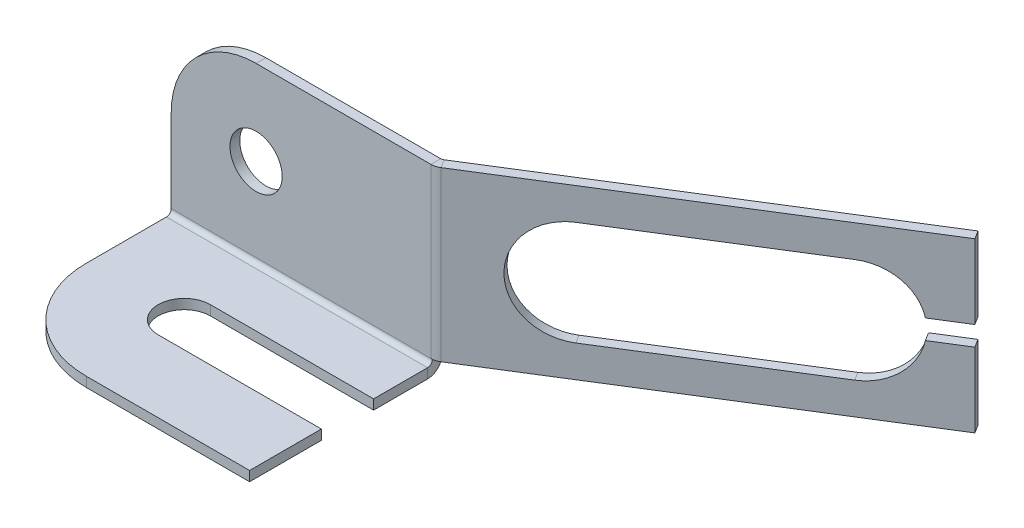
ISO-10303-21;
HEADER;
FILE_DESCRIPTION(('STEP AP214'),'2;1');
FILE_NAME('part.step','',(''),(''),'','','');
FILE_SCHEMA(('AUTOMOTIVE_DESIGN { 1 0 10303 214 1 1 1 1 }'));
ENDSEC;
DATA;
#1=APPLICATION_CONTEXT('core data for automotive mechanical design processes');
#2=APPLICATION_PROTOCOL_DEFINITION('international standard','automotive_design',2000,#1);
#3=PRODUCT_CONTEXT('',#1,'mechanical');
#4=PRODUCT('Part','Part','',(#3));
#5=PRODUCT_RELATED_PRODUCT_CATEGORY('part','',(#4));
#6=PRODUCT_DEFINITION_FORMATION('','',#4);
#7=PRODUCT_DEFINITION_CONTEXT('part definition',#1,'design');
#8=PRODUCT_DEFINITION('design','',#6,#7);
#9=PRODUCT_DEFINITION_SHAPE('','',#8);
#10=(LENGTH_UNIT() NAMED_UNIT(*) SI_UNIT(.MILLI.,.METRE.));
#11=(NAMED_UNIT(*) PLANE_ANGLE_UNIT() SI_UNIT($,.RADIAN.));
#12=(NAMED_UNIT(*) SI_UNIT($,.STERADIAN.) SOLID_ANGLE_UNIT());
#13=UNCERTAINTY_MEASURE_WITH_UNIT(LENGTH_MEASURE(1.E-05),#10,'distance_accuracy_value','');
#14=(GEOMETRIC_REPRESENTATION_CONTEXT(3) GLOBAL_UNCERTAINTY_ASSIGNED_CONTEXT((#13)) GLOBAL_UNIT_ASSIGNED_CONTEXT((#10,
#11,#12)) REPRESENTATION_CONTEXT('',''));
#15=CARTESIAN_POINT('',(0.,0.,0.));
#16=DIRECTION('',(0.,0.,1.));
#17=DIRECTION('',(1.,0.,0.));
#18=AXIS2_PLACEMENT_3D('',#15,#16,#17);
#19=CARTESIAN_POINT('',(91.3130038480239,0.736599999999992,-31.795155853992));
#20=DIRECTION('',(0.848048096156429,0.,-0.5299192642332));
#21=DIRECTION('',(-0.5299192642332,0.,-0.848048096156429));
#22=AXIS2_PLACEMENT_3D('',#19,#20,#21);
#23=PLANE('',#22);
#24=DIRECTION('',(0.5299192642332,0.,0.848048096156429));
#25=VECTOR('',#24,1.);
#26=CARTESIAN_POINT('',(91.3130038480239,15.1183,-31.795155853992));
#27=LINE('',#26,#25);
#28=CARTESIAN_POINT('',(90.5181249516741,15.1183,-33.0672279982266));
#29=VERTEX_POINT('',#28);
#30=CARTESIAN_POINT('',(91.3130038480239,15.1183,-31.795155853992));
#31=VERTEX_POINT('',#30);
#32=EDGE_CURVE('E463',#29,#31,#27,.T.);
#33=ORIENTED_EDGE('',*,*,#32,.F.);
#34=DIRECTION('',(0.,-1.,0.));
#35=VECTOR('',#34,1.);
#36=CARTESIAN_POINT('',(90.5181249516741,0.736599999999992,-33.0672279982266));
#37=LINE('',#36,#35);
#38=CARTESIAN_POINT('',(90.5181249516741,26.5,-33.0672279982266));
#39=VERTEX_POINT('',#38);
#40=EDGE_CURVE('E284',#39,#29,#37,.T.);
#41=ORIENTED_EDGE('',*,*,#40,.F.);
#42=DIRECTION('',(-0.5299192642332,0.,-0.848048096156429));
#43=VECTOR('',#42,1.);
#44=CARTESIAN_POINT('',(91.3130038480239,26.5,-31.795155853992));
#45=LINE('',#44,#43);
#46=CARTESIAN_POINT('',(91.3130038480239,26.5,-31.795155853992));
#47=VERTEX_POINT('',#46);
#48=EDGE_CURVE('E283',#47,#39,#45,.T.);
#49=ORIENTED_EDGE('',*,*,#48,.F.);
#50=DIRECTION('',(0.,-1.,0.));
#51=VECTOR('',#50,1.);
#52=CARTESIAN_POINT('',(91.3130038480239,0.736599999999992,-31.795155853992));
#53=LINE('',#52,#51);
#54=EDGE_CURVE('E273',#47,#31,#53,.T.);
#55=ORIENTED_EDGE('',*,*,#54,.T.);
#56=EDGE_LOOP('',(#33,#41,#49,#55));
#57=FACE_BOUND('',#56,.T.);
#58=ADVANCED_FACE('F43',(#57),#23,.T.);
#59=CARTESIAN_POINT('',(74.6850205560978,13.6183,-33.196622744428));
#60=DIRECTION('',(0.5299192642332,0.,0.848048096156429));
#61=DIRECTION('',(0.848048096156429,0.,-0.5299192642332));
#62=AXIS2_PLACEMENT_3D('',#59,#60,#61);
#63=CYLINDRICAL_SURFACE('',#62,8.00000000000001);
#64=CARTESIAN_POINT('',(79.18933430208,13.6183,-25.9882139270984));
#65=DIRECTION('',(0.5299192642332,0.,0.848048096156429));
#66=DIRECTION('',(0.848048096156429,0.,-0.5299192642332));
#67=AXIS2_PLACEMENT_3D('',#64,#65,#66);
#68=CIRCLE('',#67,8.00000000000001);
#69=CARTESIAN_POINT('',(85.8533953129887,15.1183,-30.152381412069));
#70=VERTEX_POINT('',#69);
#71=CARTESIAN_POINT('',(79.18933430208,21.6183,-25.9882139270984));
#72=VERTEX_POINT('',#71);
#73=EDGE_CURVE('E438',#70,#72,#68,.T.);
#74=ORIENTED_EDGE('',*,*,#73,.F.);
#75=DIRECTION('',(0.5299192642332,0.,0.848048096156429));
#76=VECTOR('',#75,1.);
#77=CARTESIAN_POINT('',(81.3490815670065,15.1183,-37.3607902293987));
#78=LINE('',#77,#76);
#79=CARTESIAN_POINT('',(86.6482742093385,15.1183,-28.8803092678344));
#80=VERTEX_POINT('',#79);
#81=EDGE_CURVE('E11',#70,#80,#78,.T.);
#82=ORIENTED_EDGE('',*,*,#81,.T.);
#83=CARTESIAN_POINT('',(79.9842131984298,13.6183,-24.7161417828637));
#84=DIRECTION('',(0.5299192642332,0.,0.848048096156429));
#85=DIRECTION('',(0.848048096156429,0.,-0.5299192642332));
#86=AXIS2_PLACEMENT_3D('',#83,#84,#85);
#87=CIRCLE('',#86,8.00000000000001);
#88=CARTESIAN_POINT('',(79.9842131984298,21.6183,-24.7161417828637));
#89=VERTEX_POINT('',#88);
#90=EDGE_CURVE('E243',#80,#89,#87,.T.);
#91=ORIENTED_EDGE('',*,*,#90,.T.);
#92=DIRECTION('',(0.5299192642332,0.,0.848048096156429));
#93=VECTOR('',#92,1.);
#94=CARTESIAN_POINT('',(74.6850205560978,21.6183,-33.196622744428));
#95=LINE('',#94,#93);
#96=EDGE_CURVE('E253',#72,#89,#95,.T.);
#97=ORIENTED_EDGE('',*,*,#96,.F.);
#98=EDGE_LOOP('',(#74,#82,#91,#97));
#99=FACE_BOUND('',#98,.T.);
#100=ADVANCED_FACE('F489',(#99),#63,.F.);
#101=CARTESIAN_POINT('',(40.,0.736599999999992,-1.5));
#102=DIRECTION('',(0.,1.,0.));
#103=DIRECTION('',(-1.,0.,0.));
#104=AXIS2_PLACEMENT_3D('',#101,#102,#103);
#105=PLANE('',#104);
#106=DIRECTION('',(0.,0.,-1.));
#107=VECTOR('',#106,1.);
#108=CARTESIAN_POINT('',(40.,0.736599999999997,0.));
#109=LINE('',#108,#107);
#110=CARTESIAN_POINT('',(40.,0.736599999999992,0.));
#111=VERTEX_POINT('',#110);
#112=CARTESIAN_POINT('',(40.,0.736599999999997,-0.00999561523000589));
#113=VERTEX_POINT('',#112);
#114=EDGE_CURVE('E333',#111,#113,#109,.T.);
#115=ORIENTED_EDGE('',*,*,#114,.T.);
#116=CARTESIAN_POINT('',(39.7887833488501,0.736599999999994,-2.23659999999999));
#117=DIRECTION('',(0.,-1.,0.));
#118=DIRECTION('',(0.,0.,-1.));
#119=AXIS2_PLACEMENT_3D('',#116,#117,#118);
#120=CIRCLE('',#119,2.23659999999998);
#121=CARTESIAN_POINT('',(39.7887833488501,0.736599999999997,0.));
#122=VERTEX_POINT('',#121);
#123=EDGE_CURVE('E306',#113,#122,#120,.T.);
#124=ORIENTED_EDGE('',*,*,#123,.T.);
#125=DIRECTION('',(-1.,0.,0.));
#126=VECTOR('',#125,1.);
#127=CARTESIAN_POINT('',(40.,0.736599999999997,0.));
#128=LINE('',#127,#126);
#129=EDGE_CURVE('E324',#111,#122,#128,.T.);
#130=ORIENTED_EDGE('',*,*,#129,.F.);
#131=EDGE_LOOP('',(#115,#124,#130));
#132=FACE_BOUND('',#131,.T.);
#133=ADVANCED_FACE('F590',(#132),#105,.T.);
#134=CARTESIAN_POINT('',(0.,0.,-1.5));
#135=DIRECTION('',(0.,0.,-1.));
#136=DIRECTION('',(-1.,0.,0.));
#137=AXIS2_PLACEMENT_3D('',#134,#135,#136);
#138=PLANE('',#137);
#139=CARTESIAN_POINT('',(13.,13.5,-1.5));
#140=DIRECTION('',(0.,0.,-1.));
#141=DIRECTION('',(-1.,0.,0.));
#142=AXIS2_PLACEMENT_3D('',#139,#140,#141);
#143=CIRCLE('',#142,4.);
#144=CARTESIAN_POINT('',(9.,13.5,-1.5));
#145=VERTEX_POINT('',#144);
#146=EDGE_CURVE('E316',#145,#145,#143,.T.);
#147=ORIENTED_EDGE('',*,*,#146,.F.);
#148=EDGE_LOOP('',(#147));
#149=FACE_BOUND('',#148,.T.);
#150=DIRECTION('',(-1.,0.,0.));
#151=VECTOR('',#150,1.);
#152=CARTESIAN_POINT('',(0.,26.5,-1.5));
#153=LINE('',#152,#151);
#154=CARTESIAN_POINT('',(39.7887833488501,26.5,-1.5));
#155=VERTEX_POINT('',#154);
#156=CARTESIAN_POINT('',(13.,26.5,-1.5));
#157=VERTEX_POINT('',#156);
#158=EDGE_CURVE('E336',#155,#157,#153,.T.);
#159=ORIENTED_EDGE('',*,*,#158,.F.);
#160=DIRECTION('',(0.,-1.,0.));
#161=VECTOR('',#160,1.);
#162=CARTESIAN_POINT('',(39.7887833488501,0.736599999999993,-1.50000000000001));
#163=LINE('',#162,#161);
#164=CARTESIAN_POINT('',(39.7887833488501,0.736599999999993,-1.50000000000001));
#165=VERTEX_POINT('',#164);
#166=EDGE_CURVE('E307',#165,#155,#163,.F.);
#167=ORIENTED_EDGE('',*,*,#166,.F.);
#168=DIRECTION('',(-1.,0.,0.));
#169=VECTOR('',#168,1.);
#170=CARTESIAN_POINT('',(0.,0.736600000000008,-1.5));
#171=LINE('',#170,#169);
#172=CARTESIAN_POINT('',(0.,0.736600000000008,-1.5));
#173=VERTEX_POINT('',#172);
#174=EDGE_CURVE('E328',#165,#173,#171,.T.);
#175=ORIENTED_EDGE('',*,*,#174,.T.);
#176=DIRECTION('',(0.,-1.,0.));
#177=VECTOR('',#176,1.);
#178=CARTESIAN_POINT('',(0.,0.,-1.5));
#179=LINE('',#178,#177);
#180=CARTESIAN_POINT('',(0.,13.5,-1.5));
#181=VERTEX_POINT('',#180);
#182=EDGE_CURVE('E338',#181,#173,#179,.T.);
#183=ORIENTED_EDGE('',*,*,#182,.F.);
#184=CARTESIAN_POINT('',(13.,13.5,-1.5));
#185=DIRECTION('',(0.,0.,-1.));
#186=DIRECTION('',(-1.,0.,0.));
#187=AXIS2_PLACEMENT_3D('',#184,#185,#186);
#188=CIRCLE('',#187,13.);
#189=EDGE_CURVE('E435',#181,#157,#188,.T.);
#190=ORIENTED_EDGE('',*,*,#189,.T.);
#191=EDGE_LOOP('',(#159,#167,#175,#183,#190));
#192=FACE_BOUND('',#191,.T.);
#193=ADVANCED_FACE('F502',(#149,#192),#138,.T.);
#194=CARTESIAN_POINT('',(0.,0.,0.));
#195=DIRECTION('',(0.,0.,-1.));
#196=DIRECTION('',(-1.,0.,0.));
#197=AXIS2_PLACEMENT_3D('',#194,#195,#196);
#198=PLANE('',#197);
#199=CARTESIAN_POINT('',(13.,13.5,0.));
#200=DIRECTION('',(0.,0.,1.));
#201=DIRECTION('',(1.,0.,0.));
#202=AXIS2_PLACEMENT_3D('',#199,#200,#201);
#203=CIRCLE('',#202,4.);
#204=CARTESIAN_POINT('',(17.,13.5,0.));
#205=VERTEX_POINT('',#204);
#206=EDGE_CURVE('E317',#205,#205,#203,.T.);
#207=ORIENTED_EDGE('',*,*,#206,.F.);
#208=EDGE_LOOP('',(#207));
#209=FACE_BOUND('',#208,.T.);
#210=DIRECTION('',(0.,-1.,0.));
#211=VECTOR('',#210,1.);
#212=CARTESIAN_POINT('',(39.7887833488501,0.736599999999993,0.));
#213=LINE('',#212,#211);
#214=CARTESIAN_POINT('',(39.7887833488501,26.5,0.));
#215=VERTEX_POINT('',#214);
#216=EDGE_CURVE('E294',#122,#215,#213,.F.);
#217=ORIENTED_EDGE('',*,*,#216,.T.);
#218=DIRECTION('',(-1.,0.,0.));
#219=VECTOR('',#218,1.);
#220=CARTESIAN_POINT('',(0.,26.5,0.));
#221=LINE('',#220,#219);
#222=CARTESIAN_POINT('',(13.,26.5,0.));
#223=VERTEX_POINT('',#222);
#224=EDGE_CURVE('E340',#215,#223,#221,.T.);
#225=ORIENTED_EDGE('',*,*,#224,.T.);
#226=CARTESIAN_POINT('',(13.,13.5,0.));
#227=DIRECTION('',(0.,0.,-1.));
#228=DIRECTION('',(-1.,0.,0.));
#229=AXIS2_PLACEMENT_3D('',#226,#227,#228);
#230=CIRCLE('',#229,13.);
#231=CARTESIAN_POINT('',(0.,13.5,0.));
#232=VERTEX_POINT('',#231);
#233=EDGE_CURVE('E426',#223,#232,#230,.F.);
#234=ORIENTED_EDGE('',*,*,#233,.T.);
#235=DIRECTION('',(0.,-1.,0.));
#236=VECTOR('',#235,1.);
#237=CARTESIAN_POINT('',(0.,0.,0.));
#238=LINE('',#237,#236);
#239=CARTESIAN_POINT('',(0.,0.736599999999992,0.));
#240=VERTEX_POINT('',#239);
#241=EDGE_CURVE('E342',#232,#240,#238,.T.);
#242=ORIENTED_EDGE('',*,*,#241,.T.);
#243=EDGE_CURVE('E329',#122,#240,#128,.T.);
#244=ORIENTED_EDGE('',*,*,#243,.F.);
#245=EDGE_LOOP('',(#217,#225,#234,#242,#244));
#246=FACE_BOUND('',#245,.T.);
#247=ADVANCED_FACE('F628',(#209,#246),#198,.F.);
#248=CARTESIAN_POINT('',(0.,-1.5,0.));
#249=DIRECTION('',(-1.,0.,0.));
#250=DIRECTION('',(0.,0.,1.));
#251=AXIS2_PLACEMENT_3D('',#248,#249,#250);
#252=PLANE('',#251);
#253=DIRECTION('',(0.,0.,1.));
#254=VECTOR('',#253,1.);
#255=CARTESIAN_POINT('',(0.,0.,0.));
#256=LINE('',#255,#254);
#257=CARTESIAN_POINT('',(0.,0.,0.736599999999999));
#258=VERTEX_POINT('',#257);
#259=CARTESIAN_POINT('',(0.,0.,13.));
#260=VERTEX_POINT('',#259);
#261=EDGE_CURVE('E398',#258,#260,#256,.T.);
#262=ORIENTED_EDGE('',*,*,#261,.F.);
#263=DIRECTION('',(0.,-1.,0.));
#264=VECTOR('',#263,1.);
#265=CARTESIAN_POINT('',(0.,0.,0.736599999999999));
#266=LINE('',#265,#264);
#267=CARTESIAN_POINT('',(0.,-1.50000000000001,0.736599999999999));
#268=VERTEX_POINT('',#267);
#269=EDGE_CURVE('E352',#258,#268,#266,.T.);
#270=ORIENTED_EDGE('',*,*,#269,.T.);
#271=DIRECTION('',(0.,0.,1.));
#272=VECTOR('',#271,1.);
#273=CARTESIAN_POINT('',(0.,-1.5,0.));
#274=LINE('',#273,#272);
#275=CARTESIAN_POINT('',(0.,-1.5,13.));
#276=VERTEX_POINT('',#275);
#277=EDGE_CURVE('E400',#268,#276,#274,.T.);
#278=ORIENTED_EDGE('',*,*,#277,.T.);
#279=DIRECTION('',(0.,1.,0.));
#280=VECTOR('',#279,1.);
#281=CARTESIAN_POINT('',(0.,-1.5,13.));
#282=LINE('',#281,#280);
#283=EDGE_CURVE('E412',#276,#260,#282,.T.);
#284=ORIENTED_EDGE('',*,*,#283,.T.);
#285=EDGE_LOOP('',(#262,#270,#278,#284));
#286=FACE_BOUND('',#285,.T.);
#287=ADVANCED_FACE('F553',(#286),#252,.T.);
#288=CARTESIAN_POINT('',(0.,-1.5,0.));
#289=DIRECTION('',(0.,1.,0.));
#290=DIRECTION('',(0.,0.,1.));
#291=AXIS2_PLACEMENT_3D('',#288,#289,#290);
#292=PLANE('',#291);
#293=DIRECTION('',(-1.,0.,0.));
#294=VECTOR('',#293,1.);
#295=CARTESIAN_POINT('',(0.,-1.50000000000001,0.736599999999999));
#296=LINE('',#295,#294);
#297=CARTESIAN_POINT('',(40.,-1.5,0.736599999999999));
#298=VERTEX_POINT('',#297);
#299=EDGE_CURVE('E346',#268,#298,#296,.F.);
#300=ORIENTED_EDGE('',*,*,#299,.T.);
#301=DIRECTION('',(0.,0.,-1.));
#302=VECTOR('',#301,1.);
#303=CARTESIAN_POINT('',(40.,-1.5,0.));
#304=LINE('',#303,#302);
#305=CARTESIAN_POINT('',(40.,-1.5,9.));
#306=VERTEX_POINT('',#305);
#307=EDGE_CURVE('E405',#306,#298,#304,.T.);
#308=ORIENTED_EDGE('',*,*,#307,.F.);
#309=DIRECTION('',(-1.,0.,0.));
#310=VECTOR('',#309,1.);
#311=CARTESIAN_POINT('',(0.,-1.5,9.));
#312=LINE('',#311,#310);
#313=CARTESIAN_POINT('',(15.,-1.5,9.));
#314=VERTEX_POINT('',#313);
#315=EDGE_CURVE('E388',#306,#314,#312,.T.);
#316=ORIENTED_EDGE('',*,*,#315,.T.);
#317=CARTESIAN_POINT('',(15.,-1.5,13.));
#318=DIRECTION('',(0.,1.,0.));
#319=DIRECTION('',(0.,0.,1.));
#320=AXIS2_PLACEMENT_3D('',#317,#318,#319);
#321=CIRCLE('',#320,4.);
#322=CARTESIAN_POINT('',(15.,-1.5,17.));
#323=VERTEX_POINT('',#322);
#324=EDGE_CURVE('E395',#314,#323,#321,.T.);
#325=ORIENTED_EDGE('',*,*,#324,.T.);
#326=DIRECTION('',(1.,0.,0.));
#327=VECTOR('',#326,1.);
#328=CARTESIAN_POINT('',(0.,-1.5,17.));
#329=LINE('',#328,#327);
#330=CARTESIAN_POINT('',(40.,-1.5,17.));
#331=VERTEX_POINT('',#330);
#332=EDGE_CURVE('E379',#323,#331,#329,.T.);
#333=ORIENTED_EDGE('',*,*,#332,.T.);
#334=CARTESIAN_POINT('',(40.,-1.5,28.));
#335=VERTEX_POINT('',#334);
#336=EDGE_CURVE('E401',#335,#331,#304,.T.);
#337=ORIENTED_EDGE('',*,*,#336,.F.);
#338=DIRECTION('',(1.,0.,0.));
#339=VECTOR('',#338,1.);
#340=CARTESIAN_POINT('',(0.,-1.5,28.));
#341=LINE('',#340,#339);
#342=CARTESIAN_POINT('',(15.,-1.5,28.));
#343=VERTEX_POINT('',#342);
#344=EDGE_CURVE('E399',#343,#335,#341,.T.);
#345=ORIENTED_EDGE('',*,*,#344,.F.);
#346=CARTESIAN_POINT('',(15.,-1.5,13.));
#347=DIRECTION('',(0.,1.,0.));
#348=DIRECTION('',(0.,0.,1.));
#349=AXIS2_PLACEMENT_3D('',#346,#347,#348);
#350=CIRCLE('',#349,15.);
#351=EDGE_CURVE('E422',#343,#276,#350,.F.);
#352=ORIENTED_EDGE('',*,*,#351,.T.);
#353=ORIENTED_EDGE('',*,*,#277,.F.);
#354=EDGE_LOOP('',(#300,#308,#316,#325,#333,#337,#345,#352,#353));
#355=FACE_BOUND('',#354,.T.);
#356=ADVANCED_FACE('F546',(#355),#292,.F.);
#357=CARTESIAN_POINT('',(0.,0.,0.));
#358=DIRECTION('',(0.,1.,0.));
#359=DIRECTION('',(0.,0.,1.));
#360=AXIS2_PLACEMENT_3D('',#357,#358,#359);
#361=PLANE('',#360);
#362=DIRECTION('',(0.,0.,-1.));
#363=VECTOR('',#362,1.);
#364=CARTESIAN_POINT('',(40.,0.,0.));
#365=LINE('',#364,#363);
#366=CARTESIAN_POINT('',(40.,0.,9.));
#367=VERTEX_POINT('',#366);
#368=CARTESIAN_POINT('',(40.,0.,0.736599999999999));
#369=VERTEX_POINT('',#368);
#370=EDGE_CURVE('E408',#367,#369,#365,.T.);
#371=ORIENTED_EDGE('',*,*,#370,.T.);
#372=DIRECTION('',(-1.,0.,0.));
#373=VECTOR('',#372,1.);
#374=CARTESIAN_POINT('',(0.,0.,0.736599999999999));
#375=LINE('',#374,#373);
#376=EDGE_CURVE('E359',#258,#369,#375,.F.);
#377=ORIENTED_EDGE('',*,*,#376,.F.);
#378=ORIENTED_EDGE('',*,*,#261,.T.);
#379=CARTESIAN_POINT('',(15.,0.,13.));
#380=DIRECTION('',(0.,1.,0.));
#381=DIRECTION('',(0.,0.,1.));
#382=AXIS2_PLACEMENT_3D('',#379,#380,#381);
#383=CIRCLE('',#382,15.);
#384=CARTESIAN_POINT('',(15.,0.,28.));
#385=VERTEX_POINT('',#384);
#386=EDGE_CURVE('E418',#260,#385,#383,.T.);
#387=ORIENTED_EDGE('',*,*,#386,.T.);
#388=DIRECTION('',(1.,0.,0.));
#389=VECTOR('',#388,1.);
#390=CARTESIAN_POINT('',(0.,0.,28.));
#391=LINE('',#390,#389);
#392=CARTESIAN_POINT('',(40.,0.,28.));
#393=VERTEX_POINT('',#392);
#394=EDGE_CURVE('E409',#385,#393,#391,.T.);
#395=ORIENTED_EDGE('',*,*,#394,.T.);
#396=CARTESIAN_POINT('',(40.,0.,17.));
#397=VERTEX_POINT('',#396);
#398=EDGE_CURVE('E397',#393,#397,#365,.T.);
#399=ORIENTED_EDGE('',*,*,#398,.T.);
#400=DIRECTION('',(1.,0.,0.));
#401=VECTOR('',#400,1.);
#402=CARTESIAN_POINT('',(15.,0.,17.));
#403=LINE('',#402,#401);
#404=CARTESIAN_POINT('',(15.,0.,17.));
#405=VERTEX_POINT('',#404);
#406=EDGE_CURVE('E375',#405,#397,#403,.T.);
#407=ORIENTED_EDGE('',*,*,#406,.F.);
#408=CARTESIAN_POINT('',(15.,0.,13.));
#409=DIRECTION('',(0.,1.,0.));
#410=DIRECTION('',(0.,0.,1.));
#411=AXIS2_PLACEMENT_3D('',#408,#409,#410);
#412=CIRCLE('',#411,4.);
#413=CARTESIAN_POINT('',(15.,0.,9.));
#414=VERTEX_POINT('',#413);
#415=EDGE_CURVE('E368',#414,#405,#412,.T.);
#416=ORIENTED_EDGE('',*,*,#415,.F.);
#417=DIRECTION('',(-1.,0.,0.));
#418=VECTOR('',#417,1.);
#419=CARTESIAN_POINT('',(15.,0.,9.));
#420=LINE('',#419,#418);
#421=EDGE_CURVE('E372',#367,#414,#420,.T.);
#422=ORIENTED_EDGE('',*,*,#421,.F.);
#423=EDGE_LOOP('',(#371,#377,#378,#387,#395,#399,#407,#416,#422));
#424=FACE_BOUND('',#423,.T.);
#425=ADVANCED_FACE('F529',(#424),#361,.T.);
#426=CARTESIAN_POINT('',(40.,-1.5,0.));
#427=DIRECTION('',(1.,0.,0.));
#428=DIRECTION('',(0.,0.,-1.));
#429=AXIS2_PLACEMENT_3D('',#426,#427,#428);
#430=PLANE('',#429);
#431=DIRECTION('',(0.,-1.,0.));
#432=VECTOR('',#431,1.);
#433=CARTESIAN_POINT('',(40.,0.,0.736599999999999));
#434=LINE('',#433,#432);
#435=EDGE_CURVE('E362',#369,#298,#434,.T.);
#436=ORIENTED_EDGE('',*,*,#435,.F.);
#437=ORIENTED_EDGE('',*,*,#370,.F.);
#438=DIRECTION('',(0.,1.,0.));
#439=VECTOR('',#438,1.);
#440=CARTESIAN_POINT('',(40.,-10.,9.));
#441=LINE('',#440,#439);
#442=EDGE_CURVE('E382',#306,#367,#441,.T.);
#443=ORIENTED_EDGE('',*,*,#442,.F.);
#444=ORIENTED_EDGE('',*,*,#307,.T.);
#445=EDGE_LOOP('',(#436,#437,#443,#444));
#446=FACE_BOUND('',#445,.T.);
#447=ADVANCED_FACE('F521',(#446),#430,.T.);
#448=DIRECTION('',(0.,1.,0.));
#449=VECTOR('',#448,1.);
#450=CARTESIAN_POINT('',(40.,-10.,17.));
#451=LINE('',#450,#449);
#452=EDGE_CURVE('E384',#331,#397,#451,.T.);
#453=ORIENTED_EDGE('',*,*,#452,.T.);
#454=ORIENTED_EDGE('',*,*,#398,.F.);
#455=DIRECTION('',(0.,1.,0.));
#456=VECTOR('',#455,1.);
#457=CARTESIAN_POINT('',(40.,-1.5,28.));
#458=LINE('',#457,#456);
#459=EDGE_CURVE('E407',#335,#393,#458,.T.);
#460=ORIENTED_EDGE('',*,*,#459,.F.);
#461=ORIENTED_EDGE('',*,*,#336,.T.);
#462=EDGE_LOOP('',(#453,#454,#460,#461));
#463=FACE_BOUND('',#462,.T.);
#464=ADVANCED_FACE('F565',(#463),#430,.T.);
#465=CARTESIAN_POINT('',(0.,-1.5,28.));
#466=DIRECTION('',(0.,0.,1.));
#467=DIRECTION('',(1.,0.,0.));
#468=AXIS2_PLACEMENT_3D('',#465,#466,#467);
#469=PLANE('',#468);
#470=ORIENTED_EDGE('',*,*,#394,.F.);
#471=DIRECTION('',(0.,1.,0.));
#472=VECTOR('',#471,1.);
#473=CARTESIAN_POINT('',(15.,-1.5,28.));
#474=LINE('',#473,#472);
#475=EDGE_CURVE('E419',#385,#343,#474,.F.);
#476=ORIENTED_EDGE('',*,*,#475,.T.);
#477=ORIENTED_EDGE('',*,*,#344,.T.);
#478=ORIENTED_EDGE('',*,*,#459,.T.);
#479=EDGE_LOOP('',(#470,#476,#477,#478));
#480=FACE_BOUND('',#479,.T.);
#481=ADVANCED_FACE('F556',(#480),#469,.T.);
#482=CARTESIAN_POINT('',(15.,-1.5,13.));
#483=DIRECTION('',(0.,1.,0.));
#484=DIRECTION('',(0.,0.,1.));
#485=AXIS2_PLACEMENT_3D('',#482,#483,#484);
#486=CYLINDRICAL_SURFACE('',#485,15.);
#487=ORIENTED_EDGE('',*,*,#351,.F.);
#488=ORIENTED_EDGE('',*,*,#475,.F.);
#489=ORIENTED_EDGE('',*,*,#386,.F.);
#490=ORIENTED_EDGE('',*,*,#283,.F.);
#491=EDGE_LOOP('',(#487,#488,#489,#490));
#492=FACE_BOUND('',#491,.T.);
#493=ADVANCED_FACE('F558',(#492),#486,.T.);
#494=CARTESIAN_POINT('',(15.,-10.,13.));
#495=DIRECTION('',(0.,1.,0.));
#496=DIRECTION('',(0.,0.,1.));
#497=AXIS2_PLACEMENT_3D('',#494,#495,#496);
#498=CYLINDRICAL_SURFACE('',#497,4.);
#499=DIRECTION('',(0.,1.,0.));
#500=VECTOR('',#499,1.);
#501=CARTESIAN_POINT('',(15.,-10.,9.));
#502=LINE('',#501,#500);
#503=EDGE_CURVE('E377',#314,#414,#502,.T.);
#504=ORIENTED_EDGE('',*,*,#503,.T.);
#505=ORIENTED_EDGE('',*,*,#415,.T.);
#506=DIRECTION('',(0.,1.,0.));
#507=VECTOR('',#506,1.);
#508=CARTESIAN_POINT('',(15.,-10.,17.));
#509=LINE('',#508,#507);
#510=EDGE_CURVE('E380',#323,#405,#509,.T.);
#511=ORIENTED_EDGE('',*,*,#510,.F.);
#512=ORIENTED_EDGE('',*,*,#324,.F.);
#513=EDGE_LOOP('',(#504,#505,#511,#512));
#514=FACE_BOUND('',#513,.T.);
#515=ADVANCED_FACE('F567',(#514),#498,.F.);
#516=CARTESIAN_POINT('',(15.,-10.,9.));
#517=DIRECTION('',(0.,0.,-1.));
#518=DIRECTION('',(-1.,0.,0.));
#519=AXIS2_PLACEMENT_3D('',#516,#517,#518);
#520=PLANE('',#519);
#521=ORIENTED_EDGE('',*,*,#442,.T.);
#522=ORIENTED_EDGE('',*,*,#421,.T.);
#523=ORIENTED_EDGE('',*,*,#503,.F.);
#524=ORIENTED_EDGE('',*,*,#315,.F.);
#525=EDGE_LOOP('',(#521,#522,#523,#524));
#526=FACE_BOUND('',#525,.T.);
#527=ADVANCED_FACE('F575',(#526),#520,.F.);
#528=CARTESIAN_POINT('',(15.,-10.,17.));
#529=DIRECTION('',(0.,0.,1.));
#530=DIRECTION('',(1.,0.,0.));
#531=AXIS2_PLACEMENT_3D('',#528,#529,#530);
#532=PLANE('',#531);
#533=ORIENTED_EDGE('',*,*,#510,.T.);
#534=ORIENTED_EDGE('',*,*,#406,.T.);
#535=ORIENTED_EDGE('',*,*,#452,.F.);
#536=ORIENTED_EDGE('',*,*,#332,.F.);
#537=EDGE_LOOP('',(#533,#534,#535,#536));
#538=FACE_BOUND('',#537,.T.);
#539=ADVANCED_FACE('F566',(#538),#532,.F.);
#540=CARTESIAN_POINT('',(40.,0.736599999999992,0.736599999999999));
#541=DIRECTION('',(1.,0.,0.));
#542=DIRECTION('',(0.,0.,-1.));
#543=AXIS2_PLACEMENT_3D('',#540,#541,#542);
#544=PLANE('',#543);
#545=ORIENTED_EDGE('',*,*,#114,.F.);
#546=CARTESIAN_POINT('',(40.,0.736599999999992,0.736599999999999));
#547=DIRECTION('',(-1.,0.,0.));
#548=DIRECTION('',(0.,0.,1.));
#549=AXIS2_PLACEMENT_3D('',#546,#547,#548);
#550=CIRCLE('',#549,0.736599999999999);
#551=EDGE_CURVE('E357',#369,#111,#550,.F.);
#552=ORIENTED_EDGE('',*,*,#551,.F.);
#553=ORIENTED_EDGE('',*,*,#435,.T.);
#554=CARTESIAN_POINT('',(40.,0.736599999999992,0.736599999999999));
#555=DIRECTION('',(-1.,0.,0.));
#556=DIRECTION('',(0.,0.,1.));
#557=AXIS2_PLACEMENT_3D('',#554,#555,#556);
#558=CIRCLE('',#557,2.2366);
#559=CARTESIAN_POINT('',(40.,0.736599999999992,-1.5));
#560=VERTEX_POINT('',#559);
#561=EDGE_CURVE('E347',#298,#560,#558,.F.);
#562=ORIENTED_EDGE('',*,*,#561,.T.);
#563=EDGE_CURVE('E325',#113,#560,#109,.T.);
#564=ORIENTED_EDGE('',*,*,#563,.F.);
#565=EDGE_LOOP('',(#545,#552,#553,#562,#564));
#566=FACE_BOUND('',#565,.T.);
#567=ADVANCED_FACE('F519',(#566),#544,.T.);
#568=CARTESIAN_POINT('',(0.,0.736599999999992,0.736599999999999));
#569=DIRECTION('',(1.,0.,0.));
#570=DIRECTION('',(0.,0.,-1.));
#571=AXIS2_PLACEMENT_3D('',#568,#569,#570);
#572=PLANE('',#571);
#573=CARTESIAN_POINT('',(0.,0.736599999999992,0.736599999999999));
#574=DIRECTION('',(-1.,0.,0.));
#575=DIRECTION('',(0.,0.,1.));
#576=AXIS2_PLACEMENT_3D('',#573,#574,#575);
#577=CIRCLE('',#576,0.736599999999999);
#578=EDGE_CURVE('E341',#240,#258,#577,.T.);
#579=ORIENTED_EDGE('',*,*,#578,.F.);
#580=DIRECTION('',(0.,0.,-1.));
#581=VECTOR('',#580,1.);
#582=CARTESIAN_POINT('',(0.,0.736599999999997,0.));
#583=LINE('',#582,#581);
#584=EDGE_CURVE('E327',#240,#173,#583,.T.);
#585=ORIENTED_EDGE('',*,*,#584,.T.);
#586=CARTESIAN_POINT('',(0.,0.736599999999992,0.736599999999999));
#587=DIRECTION('',(-1.,0.,0.));
#588=DIRECTION('',(0.,0.,1.));
#589=AXIS2_PLACEMENT_3D('',#586,#587,#588);
#590=CIRCLE('',#589,2.2366);
#591=EDGE_CURVE('E351',#173,#268,#590,.T.);
#592=ORIENTED_EDGE('',*,*,#591,.T.);
#593=ORIENTED_EDGE('',*,*,#269,.F.);
#594=EDGE_LOOP('',(#579,#585,#592,#593));
#595=FACE_BOUND('',#594,.T.);
#596=ADVANCED_FACE('F538',(#595),#572,.F.);
#597=CARTESIAN_POINT('',(0.,0.736599999999992,0.736599999999999));
#598=DIRECTION('',(-1.,0.,0.));
#599=DIRECTION('',(0.,0.,-1.));
#600=AXIS2_PLACEMENT_3D('',#597,#598,#599);
#601=CYLINDRICAL_SURFACE('',#600,2.2366);
#602=ORIENTED_EDGE('',*,*,#299,.F.);
#603=ORIENTED_EDGE('',*,*,#591,.F.);
#604=ORIENTED_EDGE('',*,*,#174,.F.);
#605=EDGE_CURVE('E334',#560,#165,#171,.T.);
#606=ORIENTED_EDGE('',*,*,#605,.F.);
#607=ORIENTED_EDGE('',*,*,#561,.F.);
#608=EDGE_LOOP('',(#602,#603,#604,#606,#607));
#609=FACE_BOUND('',#608,.T.);
#610=ADVANCED_FACE('F513',(#609),#601,.T.);
#611=CARTESIAN_POINT('',(0.,0.736599999999992,0.736599999999999));
#612=DIRECTION('',(-1.,0.,0.));
#613=DIRECTION('',(0.,0.,-1.));
#614=AXIS2_PLACEMENT_3D('',#611,#612,#613);
#615=CYLINDRICAL_SURFACE('',#614,0.736599999999999);
#616=ORIENTED_EDGE('',*,*,#376,.T.);
#617=ORIENTED_EDGE('',*,*,#551,.T.);
#618=ORIENTED_EDGE('',*,*,#129,.T.);
#619=ORIENTED_EDGE('',*,*,#243,.T.);
#620=ORIENTED_EDGE('',*,*,#578,.T.);
#621=EDGE_LOOP('',(#616,#617,#618,#619,#620));
#622=FACE_BOUND('',#621,.T.);
#623=ADVANCED_FACE('F531',(#622),#615,.F.);
#624=CARTESIAN_POINT('',(0.,0.,-1.5));
#625=DIRECTION('',(-1.,0.,0.));
#626=DIRECTION('',(0.,0.,1.));
#627=AXIS2_PLACEMENT_3D('',#624,#625,#626);
#628=PLANE('',#627);
#629=ORIENTED_EDGE('',*,*,#241,.F.);
#630=DIRECTION('',(0.,0.,1.));
#631=VECTOR('',#630,1.);
#632=CARTESIAN_POINT('',(0.,13.5,-1.5));
#633=LINE('',#632,#631);
#634=EDGE_CURVE('E427',#232,#181,#633,.F.);
#635=ORIENTED_EDGE('',*,*,#634,.T.);
#636=ORIENTED_EDGE('',*,*,#182,.T.);
#637=ORIENTED_EDGE('',*,*,#584,.F.);
#638=EDGE_LOOP('',(#629,#635,#636,#637));
#639=FACE_BOUND('',#638,.T.);
#640=ADVANCED_FACE('F541',(#639),#628,.T.);
#641=CARTESIAN_POINT('',(0.,26.5,-1.5));
#642=DIRECTION('',(0.,1.,0.));
#643=DIRECTION('',(0.,0.,1.));
#644=AXIS2_PLACEMENT_3D('',#641,#642,#643);
#645=PLANE('',#644);
#646=DIRECTION('',(0.,0.,1.));
#647=VECTOR('',#646,1.);
#648=CARTESIAN_POINT('',(39.7887833488501,26.5,-1.5));
#649=LINE('',#648,#647);
#650=EDGE_CURVE('E305',#155,#215,#649,.T.);
#651=ORIENTED_EDGE('',*,*,#650,.F.);
#652=ORIENTED_EDGE('',*,*,#158,.T.);
#653=DIRECTION('',(0.,0.,1.));
#654=VECTOR('',#653,1.);
#655=CARTESIAN_POINT('',(13.,26.5,-1.5));
#656=LINE('',#655,#654);
#657=EDGE_CURVE('E424',#157,#223,#656,.T.);
#658=ORIENTED_EDGE('',*,*,#657,.T.);
#659=ORIENTED_EDGE('',*,*,#224,.F.);
#660=EDGE_LOOP('',(#651,#652,#658,#659));
#661=FACE_BOUND('',#660,.T.);
#662=ADVANCED_FACE('F501',(#661),#645,.T.);
#663=CARTESIAN_POINT('',(13.,13.5,-1.5));
#664=DIRECTION('',(0.,0.,1.));
#665=DIRECTION('',(1.,0.,0.));
#666=AXIS2_PLACEMENT_3D('',#663,#664,#665);
#667=CYLINDRICAL_SURFACE('',#666,13.);
#668=ORIENTED_EDGE('',*,*,#189,.F.);
#669=ORIENTED_EDGE('',*,*,#634,.F.);
#670=ORIENTED_EDGE('',*,*,#233,.F.);
#671=ORIENTED_EDGE('',*,*,#657,.F.);
#672=EDGE_LOOP('',(#668,#669,#670,#671));
#673=FACE_BOUND('',#672,.T.);
#674=ADVANCED_FACE('F44',(#673),#667,.T.);
#675=CARTESIAN_POINT('',(13.,13.5,-10.));
#676=DIRECTION('',(0.,0.,1.));
#677=DIRECTION('',(1.,0.,0.));
#678=AXIS2_PLACEMENT_3D('',#675,#676,#677);
#679=CYLINDRICAL_SURFACE('',#678,4.);
#680=ORIENTED_EDGE('',*,*,#146,.T.);
#681=EDGE_LOOP('',(#680));
#682=FACE_BOUND('',#681,.T.);
#683=ORIENTED_EDGE('',*,*,#206,.T.);
#684=EDGE_LOOP('',(#683));
#685=FACE_BOUND('',#684,.T.);
#686=ADVANCED_FACE('F617',(#682,#685),#679,.F.);
#687=CARTESIAN_POINT('',(39.7887833488501,26.5,-2.23659999999998));
#688=DIRECTION('',(0.,1.,0.));
#689=DIRECTION('',(0.,0.,1.));
#690=AXIS2_PLACEMENT_3D('',#687,#688,#689);
#691=PLANE('',#690);
#692=DIRECTION('',(0.5299192642332,0.,0.848048096156429));
#693=VECTOR('',#692,1.);
#694=CARTESIAN_POINT('',(40.1791218788842,26.5,-1.61192777237117));
#695=LINE('',#694,#693);
#696=CARTESIAN_POINT('',(40.1791218788842,26.5,-1.61192777237117));
#697=VERTEX_POINT('',#696);
#698=CARTESIAN_POINT('',(40.974000775234,26.5,-0.339855628136535));
#699=VERTEX_POINT('',#698);
#700=EDGE_CURVE('E251',#697,#699,#695,.T.);
#701=ORIENTED_EDGE('',*,*,#700,.F.);
#702=CARTESIAN_POINT('',(39.7887833488501,26.5,-2.23659999999998));
#703=DIRECTION('',(0.,-1.,0.));
#704=DIRECTION('',(0.,0.,-1.));
#705=AXIS2_PLACEMENT_3D('',#702,#703,#704);
#706=CIRCLE('',#705,0.736599999999978);
#707=EDGE_CURVE('E304',#155,#697,#706,.F.);
#708=ORIENTED_EDGE('',*,*,#707,.F.);
#709=ORIENTED_EDGE('',*,*,#650,.T.);
#710=CARTESIAN_POINT('',(39.7887833488501,26.5,-2.23659999999998));
#711=DIRECTION('',(0.,-1.,0.));
#712=DIRECTION('',(0.,0.,-1.));
#713=AXIS2_PLACEMENT_3D('',#710,#711,#712);
#714=CIRCLE('',#713,2.23659999999998);
#715=EDGE_CURVE('E296',#215,#699,#714,.F.);
#716=ORIENTED_EDGE('',*,*,#715,.T.);
#717=EDGE_LOOP('',(#701,#708,#709,#716));
#718=FACE_BOUND('',#717,.T.);
#719=ADVANCED_FACE('F500',(#718),#691,.T.);
#720=CARTESIAN_POINT('',(39.7887833488501,0.736599999999994,-2.23659999999999));
#721=DIRECTION('',(0.,1.,0.));
#722=DIRECTION('',(0.,0.,1.));
#723=AXIS2_PLACEMENT_3D('',#720,#721,#722);
#724=PLANE('',#723);
#725=CARTESIAN_POINT('',(40.974000775234,0.736599999999992,-0.339855628136535));
#726=VERTEX_POINT('',#725);
#727=EDGE_CURVE('E299',#726,#113,#120,.T.);
#728=ORIENTED_EDGE('',*,*,#727,.T.);
#729=ORIENTED_EDGE('',*,*,#563,.T.);
#730=ORIENTED_EDGE('',*,*,#605,.T.);
#731=CARTESIAN_POINT('',(39.7887833488501,0.736599999999994,-2.23659999999999));
#732=DIRECTION('',(0.,-1.,0.));
#733=DIRECTION('',(0.,0.,-1.));
#734=AXIS2_PLACEMENT_3D('',#731,#732,#733);
#735=CIRCLE('',#734,0.736599999999978);
#736=CARTESIAN_POINT('',(40.1791218788842,0.736599999999993,-1.61192777237118));
#737=VERTEX_POINT('',#736);
#738=EDGE_CURVE('E292',#737,#165,#735,.T.);
#739=ORIENTED_EDGE('',*,*,#738,.F.);
#740=DIRECTION('',(0.5299192642332,0.,0.848048096156429));
#741=VECTOR('',#740,1.);
#742=CARTESIAN_POINT('',(40.1791218788842,0.736599999999993,-1.61192777237117));
#743=LINE('',#742,#741);
#744=EDGE_CURVE('E265',#737,#726,#743,.T.);
#745=ORIENTED_EDGE('',*,*,#744,.T.);
#746=EDGE_LOOP('',(#728,#729,#730,#739,#745));
#747=FACE_BOUND('',#746,.T.);
#748=ADVANCED_FACE('F509',(#747),#724,.F.);
#749=CARTESIAN_POINT('',(39.7887833488501,0.736599999999993,-2.23659999999999));
#750=DIRECTION('',(0.,-1.,0.));
#751=DIRECTION('',(0.5299192642332,0.,0.848048096156429));
#752=AXIS2_PLACEMENT_3D('',#749,#750,#751);
#753=CYLINDRICAL_SURFACE('',#752,2.23659999999998);
#754=ORIENTED_EDGE('',*,*,#216,.F.);
#755=ORIENTED_EDGE('',*,*,#123,.F.);
#756=ORIENTED_EDGE('',*,*,#727,.F.);
#757=DIRECTION('',(0.,-1.,0.));
#758=VECTOR('',#757,1.);
#759=CARTESIAN_POINT('',(40.974000775234,0.,-0.339855628136529));
#760=LINE('',#759,#758);
#761=EDGE_CURVE('E268',#699,#726,#760,.T.);
#762=ORIENTED_EDGE('',*,*,#761,.F.);
#763=ORIENTED_EDGE('',*,*,#715,.F.);
#764=EDGE_LOOP('',(#754,#755,#756,#762,#763));
#765=FACE_BOUND('',#764,.T.);
#766=ADVANCED_FACE('F494',(#765),#753,.T.);
#767=CARTESIAN_POINT('',(39.7887833488501,0.736599999999993,-2.23659999999999));
#768=DIRECTION('',(0.,-1.,0.));
#769=DIRECTION('',(0.5299192642332,0.,0.848048096156429));
#770=AXIS2_PLACEMENT_3D('',#767,#768,#769);
#771=CYLINDRICAL_SURFACE('',#770,0.736599999999978);
#772=ORIENTED_EDGE('',*,*,#166,.T.);
#773=ORIENTED_EDGE('',*,*,#707,.T.);
#774=DIRECTION('',(0.,-1.,0.));
#775=VECTOR('',#774,1.);
#776=CARTESIAN_POINT('',(40.1791218788842,26.5,-1.61192777237117));
#777=LINE('',#776,#775);
#778=EDGE_CURVE('E262',#697,#737,#777,.T.);
#779=ORIENTED_EDGE('',*,*,#778,.T.);
#780=ORIENTED_EDGE('',*,*,#738,.T.);
#781=EDGE_LOOP('',(#772,#773,#779,#780));
#782=FACE_BOUND('',#781,.T.);
#783=ADVANCED_FACE('F507',(#782),#771,.F.);
#784=CARTESIAN_POINT('',(40.7948788963498,0.736599999999992,-0.227927855765354));
#785=DIRECTION('',(0.,-1.,0.));
#786=DIRECTION('',(0.,0.,-1.));
#787=AXIS2_PLACEMENT_3D('',#784,#785,#786);
#788=PLANE('',#787);
#789=DIRECTION('',(-0.848048096156429,0.,0.5299192642332));
#790=VECTOR('',#789,1.);
#791=CARTESIAN_POINT('',(40.7948788963498,0.736599999999992,-0.227927855765354));
#792=LINE('',#791,#790);
#793=CARTESIAN_POINT('',(91.3130038480239,0.736599999999992,-31.795155853992));
#794=VERTEX_POINT('',#793);
#795=EDGE_CURVE('E279',#794,#726,#792,.T.);
#796=ORIENTED_EDGE('',*,*,#795,.T.);
#797=ORIENTED_EDGE('',*,*,#744,.F.);
#798=DIRECTION('',(-0.848048096156429,0.,0.5299192642332));
#799=VECTOR('',#798,1.);
#800=CARTESIAN_POINT('',(40.,0.736599999999992,-1.5));
#801=LINE('',#800,#799);
#802=CARTESIAN_POINT('',(90.5181249516741,0.736599999999992,-33.0672279982266));
#803=VERTEX_POINT('',#802);
#804=EDGE_CURVE('E274',#803,#737,#801,.T.);
#805=ORIENTED_EDGE('',*,*,#804,.F.);
#806=DIRECTION('',(-0.5299192642332,0.,-0.848048096156429));
#807=VECTOR('',#806,1.);
#808=CARTESIAN_POINT('',(91.3130038480239,0.736599999999992,-31.795155853992));
#809=LINE('',#808,#807);
#810=EDGE_CURVE('E287',#794,#803,#809,.T.);
#811=ORIENTED_EDGE('',*,*,#810,.F.);
#812=EDGE_LOOP('',(#796,#797,#805,#811));
#813=FACE_BOUND('',#812,.T.);
#814=ADVANCED_FACE('F473',(#813),#788,.T.);
#815=CARTESIAN_POINT('',(91.3130038480239,26.5,-31.795155853992));
#816=DIRECTION('',(0.,1.,0.));
#817=DIRECTION('',(0.,0.,1.));
#818=AXIS2_PLACEMENT_3D('',#815,#816,#817);
#819=PLANE('',#818);
#820=DIRECTION('',(0.848048096156429,0.,-0.5299192642332));
#821=VECTOR('',#820,1.);
#822=CARTESIAN_POINT('',(90.5181249516741,26.5,-33.0672279982266));
#823=LINE('',#822,#821);
#824=EDGE_CURVE('E272',#697,#39,#823,.T.);
#825=ORIENTED_EDGE('',*,*,#824,.F.);
#826=ORIENTED_EDGE('',*,*,#700,.T.);
#827=DIRECTION('',(0.848048096156429,0.,-0.5299192642332));
#828=VECTOR('',#827,1.);
#829=CARTESIAN_POINT('',(91.3130038480239,26.5,-31.795155853992));
#830=LINE('',#829,#828);
#831=EDGE_CURVE('E275',#699,#47,#830,.T.);
#832=ORIENTED_EDGE('',*,*,#831,.T.);
#833=ORIENTED_EDGE('',*,*,#48,.T.);
#834=EDGE_LOOP('',(#825,#826,#832,#833));
#835=FACE_BOUND('',#834,.T.);
#836=ADVANCED_FACE('F481',(#835),#819,.T.);
#837=CARTESIAN_POINT('',(11.3533604258437,0.,18.1691747101261));
#838=DIRECTION('',(0.5299192642332,0.,0.848048096156429));
#839=DIRECTION('',(0.848048096156429,0.,-0.5299192642332));
#840=AXIS2_PLACEMENT_3D('',#837,#838,#839);
#841=PLANE('',#840);
#842=DIRECTION('',(-0.848048096156429,0.,0.5299192642332));
#843=VECTOR('',#842,1.);
#844=CARTESIAN_POINT('',(86.6482742093385,15.1183,-28.8803092678344));
#845=LINE('',#844,#843);
#846=EDGE_CURVE('E67',#31,#80,#845,.T.);
#847=ORIENTED_EDGE('',*,*,#846,.F.);
#848=ORIENTED_EDGE('',*,*,#54,.F.);
#849=ORIENTED_EDGE('',*,*,#831,.F.);
#850=ORIENTED_EDGE('',*,*,#761,.T.);
#851=ORIENTED_EDGE('',*,*,#795,.F.);
#852=CARTESIAN_POINT('',(91.3130038480239,12.1183,-31.795155853992));
#853=VERTEX_POINT('',#852);
#854=EDGE_CURVE('E240',#853,#794,#53,.T.);
#855=ORIENTED_EDGE('',*,*,#854,.F.);
#856=DIRECTION('',(0.848048096156429,0.,-0.5299192642332));
#857=VECTOR('',#856,1.);
#858=CARTESIAN_POINT('',(86.6482742093385,12.1183,-28.8803092678344));
#859=LINE('',#858,#857);
#860=CARTESIAN_POINT('',(86.6482742093385,12.1183,-28.8803092678344));
#861=VERTEX_POINT('',#860);
#862=EDGE_CURVE('E223',#861,#853,#859,.T.);
#863=ORIENTED_EDGE('',*,*,#862,.F.);
#864=CARTESIAN_POINT('',(79.9842131984298,5.6183,-24.7161417828637));
#865=VERTEX_POINT('',#864);
#866=EDGE_CURVE('E232',#865,#861,#87,.T.);
#867=ORIENTED_EDGE('',*,*,#866,.F.);
#868=DIRECTION('',(0.848048096156429,0.,-0.5299192642332));
#869=VECTOR('',#868,1.);
#870=CARTESIAN_POINT('',(53.6947222175805,5.61829999999999,-8.28864459163453));
#871=LINE('',#870,#869);
#872=CARTESIAN_POINT('',(53.6947222175805,5.61829999999999,-8.28864459163453));
#873=VERTEX_POINT('',#872);
#874=EDGE_CURVE('E247',#873,#865,#871,.T.);
#875=ORIENTED_EDGE('',*,*,#874,.F.);
#876=CARTESIAN_POINT('',(53.6947222175805,13.6183,-8.28864459163453));
#877=DIRECTION('',(0.5299192642332,0.,0.848048096156429));
#878=DIRECTION('',(0.848048096156429,0.,-0.5299192642332));
#879=AXIS2_PLACEMENT_3D('',#876,#877,#878);
#880=CIRCLE('',#879,8.00000000000001);
#881=CARTESIAN_POINT('',(53.6947222175805,21.6183,-8.28864459163453));
#882=VERTEX_POINT('',#881);
#883=EDGE_CURVE('E460',#882,#873,#880,.T.);
#884=ORIENTED_EDGE('',*,*,#883,.F.);
#885=DIRECTION('',(-0.848048096156429,0.,0.5299192642332));
#886=VECTOR('',#885,1.);
#887=CARTESIAN_POINT('',(53.6947222175805,21.6183,-8.28864459163453));
#888=LINE('',#887,#886);
#889=EDGE_CURVE('E245',#89,#882,#888,.T.);
#890=ORIENTED_EDGE('',*,*,#889,.F.);
#891=ORIENTED_EDGE('',*,*,#90,.F.);
#892=EDGE_LOOP('',(#847,#848,#849,#850,#851,#855,#863,#867,#875,#884,#890,#891));
#893=FACE_BOUND('',#892,.T.);
#894=ADVANCED_FACE('F231',(#893),#841,.T.);
#895=CARTESIAN_POINT('',(10.5584815294939,0.,16.8971025658914));
#896=DIRECTION('',(0.5299192642332,0.,0.848048096156429));
#897=DIRECTION('',(0.848048096156429,0.,-0.5299192642332));
#898=AXIS2_PLACEMENT_3D('',#895,#896,#897);
#899=PLANE('',#898);
#900=ORIENTED_EDGE('',*,*,#40,.T.);
#901=DIRECTION('',(-0.848048096156429,0.,0.5299192642332));
#902=VECTOR('',#901,1.);
#903=CARTESIAN_POINT('',(10.5584815294939,15.1183,16.8971025658914));
#904=LINE('',#903,#902);
#905=EDGE_CURVE('E456',#29,#70,#904,.T.);
#906=ORIENTED_EDGE('',*,*,#905,.T.);
#907=ORIENTED_EDGE('',*,*,#73,.T.);
#908=DIRECTION('',(-0.848048096156429,0.,0.5299192642332));
#909=VECTOR('',#908,1.);
#910=CARTESIAN_POINT('',(10.5584815294939,21.6183,16.8971025658914));
#911=LINE('',#910,#909);
#912=CARTESIAN_POINT('',(52.8998433212307,21.6183,-9.56071673586917));
#913=VERTEX_POINT('',#912);
#914=EDGE_CURVE('E441',#72,#913,#911,.T.);
#915=ORIENTED_EDGE('',*,*,#914,.T.);
#916=CARTESIAN_POINT('',(52.8998433212307,13.6183,-9.56071673586917));
#917=DIRECTION('',(0.5299192642332,0.,0.848048096156429));
#918=DIRECTION('',(0.848048096156429,0.,-0.5299192642332));
#919=AXIS2_PLACEMENT_3D('',#916,#917,#918);
#920=CIRCLE('',#919,8.00000000000001);
#921=CARTESIAN_POINT('',(52.8998433212307,5.61829999999999,-9.56071673586917));
#922=VERTEX_POINT('',#921);
#923=EDGE_CURVE('E230',#913,#922,#920,.T.);
#924=ORIENTED_EDGE('',*,*,#923,.T.);
#925=DIRECTION('',(0.848048096156429,0.,-0.5299192642332));
#926=VECTOR('',#925,1.);
#927=CARTESIAN_POINT('',(10.5584815294939,5.61829999999999,16.8971025658914));
#928=LINE('',#927,#926);
#929=CARTESIAN_POINT('',(79.18933430208,5.61829999999999,-25.9882139270984));
#930=VERTEX_POINT('',#929);
#931=EDGE_CURVE('E434',#922,#930,#928,.T.);
#932=ORIENTED_EDGE('',*,*,#931,.T.);
#933=CARTESIAN_POINT('',(85.8533953129887,12.1183,-30.152381412069));
#934=VERTEX_POINT('',#933);
#935=EDGE_CURVE('E437',#930,#934,#68,.T.);
#936=ORIENTED_EDGE('',*,*,#935,.T.);
#937=DIRECTION('',(0.848048096156429,0.,-0.5299192642332));
#938=VECTOR('',#937,1.);
#939=CARTESIAN_POINT('',(10.5584815294939,12.1183,16.8971025658914));
#940=LINE('',#939,#938);
#941=CARTESIAN_POINT('',(90.5181249516741,12.1183,-33.0672279982266));
#942=VERTEX_POINT('',#941);
#943=EDGE_CURVE('E59',#934,#942,#940,.T.);
#944=ORIENTED_EDGE('',*,*,#943,.T.);
#945=EDGE_CURVE('E281',#942,#803,#37,.T.);
#946=ORIENTED_EDGE('',*,*,#945,.T.);
#947=ORIENTED_EDGE('',*,*,#804,.T.);
#948=ORIENTED_EDGE('',*,*,#778,.F.);
#949=ORIENTED_EDGE('',*,*,#824,.T.);
#950=EDGE_LOOP('',(#900,#906,#907,#915,#924,#932,#936,#944,#946,#947,#948,#949));
#951=FACE_BOUND('',#950,.T.);
#952=ADVANCED_FACE('F447',(#951),#899,.F.);
#953=DIRECTION('',(-0.5299192642332,0.,-0.848048096156429));
#954=VECTOR('',#953,1.);
#955=CARTESIAN_POINT('',(91.3130038480239,12.1183,-31.795155853992));
#956=LINE('',#955,#954);
#957=EDGE_CURVE('E467',#853,#942,#956,.T.);
#958=ORIENTED_EDGE('',*,*,#957,.F.);
#959=ORIENTED_EDGE('',*,*,#854,.T.);
#960=ORIENTED_EDGE('',*,*,#810,.T.);
#961=ORIENTED_EDGE('',*,*,#945,.F.);
#962=EDGE_LOOP('',(#958,#959,#960,#961));
#963=FACE_BOUND('',#962,.T.);
#964=ADVANCED_FACE('F468',(#963),#23,.T.);
#965=CARTESIAN_POINT('',(48.3955295752485,13.6183,-16.7691255531988));
#966=DIRECTION('',(0.5299192642332,0.,0.848048096156429));
#967=DIRECTION('',(0.848048096156429,0.,-0.5299192642332));
#968=AXIS2_PLACEMENT_3D('',#965,#966,#967);
#969=CYLINDRICAL_SURFACE('',#968,8.00000000000001);
#970=DIRECTION('',(0.5299192642332,0.,0.848048096156429));
#971=VECTOR('',#970,1.);
#972=CARTESIAN_POINT('',(48.3955295752485,21.6183,-16.7691255531988));
#973=LINE('',#972,#971);
#974=EDGE_CURVE('E255',#913,#882,#973,.T.);
#975=ORIENTED_EDGE('',*,*,#974,.T.);
#976=ORIENTED_EDGE('',*,*,#883,.T.);
#977=DIRECTION('',(0.5299192642332,0.,0.848048096156429));
#978=VECTOR('',#977,1.);
#979=CARTESIAN_POINT('',(48.3955295752485,5.61829999999999,-16.7691255531988));
#980=LINE('',#979,#978);
#981=EDGE_CURVE('E246',#922,#873,#980,.T.);
#982=ORIENTED_EDGE('',*,*,#981,.F.);
#983=ORIENTED_EDGE('',*,*,#923,.F.);
#984=EDGE_LOOP('',(#975,#976,#982,#983));
#985=FACE_BOUND('',#984,.T.);
#986=ADVANCED_FACE('F452',(#985),#969,.F.);
#987=CARTESIAN_POINT('',(48.3955295752485,21.6183,-16.7691255531988));
#988=DIRECTION('',(0.,1.,0.));
#989=DIRECTION('',(0.,0.,1.));
#990=AXIS2_PLACEMENT_3D('',#987,#988,#989);
#991=PLANE('',#990);
#992=ORIENTED_EDGE('',*,*,#96,.T.);
#993=ORIENTED_EDGE('',*,*,#889,.T.);
#994=ORIENTED_EDGE('',*,*,#974,.F.);
#995=ORIENTED_EDGE('',*,*,#914,.F.);
#996=EDGE_LOOP('',(#992,#993,#994,#995));
#997=FACE_BOUND('',#996,.T.);
#998=ADVANCED_FACE('F454',(#997),#991,.F.);
#999=ORIENTED_EDGE('',*,*,#866,.T.);
#1000=DIRECTION('',(0.5299192642332,0.,0.848048096156429));
#1001=VECTOR('',#1000,1.);
#1002=CARTESIAN_POINT('',(81.3490815670065,12.1183,-37.3607902293987));
#1003=LINE('',#1002,#1001);
#1004=EDGE_CURVE('E51',#861,#934,#1003,.F.);
#1005=ORIENTED_EDGE('',*,*,#1004,.T.);
#1006=ORIENTED_EDGE('',*,*,#935,.F.);
#1007=DIRECTION('',(0.5299192642332,0.,0.848048096156429));
#1008=VECTOR('',#1007,1.);
#1009=CARTESIAN_POINT('',(74.6850205560978,5.6183,-33.196622744428));
#1010=LINE('',#1009,#1008);
#1011=EDGE_CURVE('E239',#930,#865,#1010,.T.);
#1012=ORIENTED_EDGE('',*,*,#1011,.T.);
#1013=EDGE_LOOP('',(#999,#1005,#1006,#1012));
#1014=FACE_BOUND('',#1013,.T.);
#1015=ADVANCED_FACE('F237',(#1014),#63,.F.);
#1016=CARTESIAN_POINT('',(48.3955295752485,5.61829999999999,-16.7691255531988));
#1017=DIRECTION('',(0.,-1.,0.));
#1018=DIRECTION('',(0.,0.,-1.));
#1019=AXIS2_PLACEMENT_3D('',#1016,#1017,#1018);
#1020=PLANE('',#1019);
#1021=ORIENTED_EDGE('',*,*,#981,.T.);
#1022=ORIENTED_EDGE('',*,*,#874,.T.);
#1023=ORIENTED_EDGE('',*,*,#1011,.F.);
#1024=ORIENTED_EDGE('',*,*,#931,.F.);
#1025=EDGE_LOOP('',(#1021,#1022,#1023,#1024));
#1026=FACE_BOUND('',#1025,.T.);
#1027=ADVANCED_FACE('F776',(#1026),#1020,.F.);
#1028=CARTESIAN_POINT('',(81.3490815670065,12.1183,-37.3607902293987));
#1029=DIRECTION('',(0.,-1.,0.));
#1030=DIRECTION('',(0.,0.,-1.));
#1031=AXIS2_PLACEMENT_3D('',#1028,#1029,#1030);
#1032=PLANE('',#1031);
#1033=ORIENTED_EDGE('',*,*,#1004,.F.);
#1034=ORIENTED_EDGE('',*,*,#862,.T.);
#1035=ORIENTED_EDGE('',*,*,#957,.T.);
#1036=ORIENTED_EDGE('',*,*,#943,.F.);
#1037=EDGE_LOOP('',(#1033,#1034,#1035,#1036));
#1038=FACE_BOUND('',#1037,.T.);
#1039=ADVANCED_FACE('F225',(#1038),#1032,.F.);
#1040=CARTESIAN_POINT('',(81.3490815670065,15.1183,-37.3607902293987));
#1041=DIRECTION('',(0.,1.,0.));
#1042=DIRECTION('',(0.,0.,1.));
#1043=AXIS2_PLACEMENT_3D('',#1040,#1041,#1042);
#1044=PLANE('',#1043);
#1045=ORIENTED_EDGE('',*,*,#32,.T.);
#1046=ORIENTED_EDGE('',*,*,#846,.T.);
#1047=ORIENTED_EDGE('',*,*,#81,.F.);
#1048=ORIENTED_EDGE('',*,*,#905,.F.);
#1049=EDGE_LOOP('',(#1045,#1046,#1047,#1048));
#1050=FACE_BOUND('',#1049,.T.);
#1051=ADVANCED_FACE('F808',(#1050),#1044,.F.);
#1052=CLOSED_SHELL('',(#58,#100,#133,#193,#247,#287,#356,#425,#447,#464,#481,#493,#515,#527,
#539,#567,#596,#610,#623,#640,#662,#674,#686,#719,#748,#766,#783,#814,#836,#894,#952,#964,#986,
#998,#1015,#1027,#1039,#1051));
#1053=MANIFOLD_SOLID_BREP('B2',#1052);
#1054=ADVANCED_BREP_SHAPE_REPRESENTATION('',(#18,#1053),#14);
#1055=SHAPE_DEFINITION_REPRESENTATION(#9,#1054);
ENDSEC;
END-ISO-10303-21;
